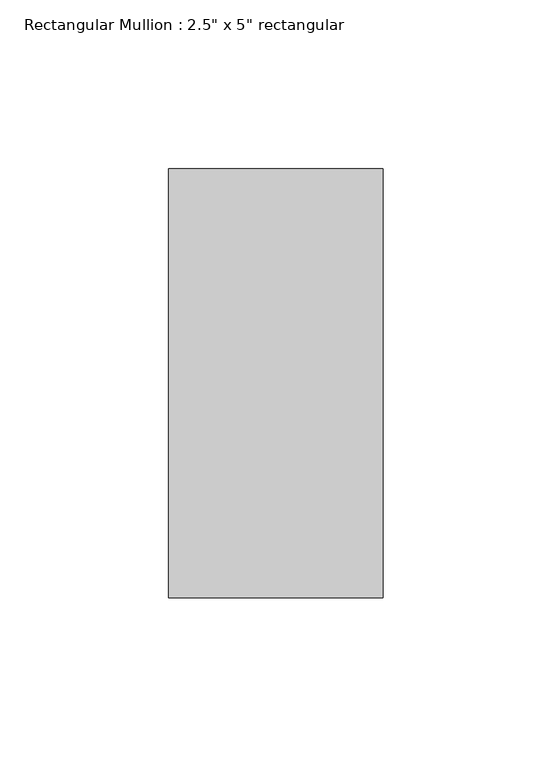
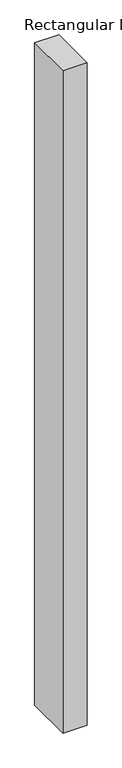
"""IFC4 building model written with IfcOpenShell, lengths in millimetres: member geometry."""

from ifc_helpers import new_model, si_unit, frame, origin, place, context, project, spatial, polyline, outline, extrude, source, transform, mapped, element, save


def member_f992ac7f(model_context):
    return source(origin(), model_context, "Body", "SweptSolid", [
        extrude(outline(polyline([(0.0, 63.5), (0.0, -63.5), (-63.5, -63.5), (-63.5, 63.5), (0.0, 63.5)])), frame((0.0, 0.0, -1825.0287468), z_axis=(0.0, 0.0, 1.0), x_axis=(1.0, 0.0, 0.0)), (0.0, 0.0, 1.0), 1825.0287468),
    ])


if __name__ == "__main__":
    model = new_model("IFC4")
    model_context = context("Model", 3, world=origin())
    ifc_project = project(units=[si_unit("LENGTHUNIT", "METRE", prefix="MILLI")], contexts=[model_context])
    site = spatial("IfcSite", under=ifc_project)
    building = spatial("IfcBuilding", under=site)
    placement = place(None, origin())
    member_shape = member_f992ac7f(model_context)
    element("IfcMember", 1, ObjectType="Rectangular Mullion : 2.5\" x 5\" rectangular", at=placement, inside=building, context=model_context, shape_type="MappedRepresentation", body=[
        mapped(member_shape, transform((0.0, 0.0, 0.0), x_axis=(1.0, 0.0, 0.0), y_axis=(0.0, 1.0, 0.0), z_axis=(0.0, 0.0, 1.0))),
    ])
    save(model, "model.ifc")

# Revit data of these elements
# Type "Rectangular Mullion : 2.5\" x 5\" rectangular"
#   built-in parameter 1007304 = 0.416667 (stored number, unit not read)
#   built-in parameter 1007301 = 0.104167 (stored number, unit not read)
#   built-in parameter 1007300 = 0.104167 (stored number, unit not read)
# Element 1 (IfcMember, "Rectangular Mullion : 2.5\" x 5\" rectangular")
#   Materials on its faces: "Aluminum"
# Materials
#   "Aluminum": class "Metal", colour RGB 247 247 247, transparency 0, Description = "Aluminum 6061", Cost = 0
